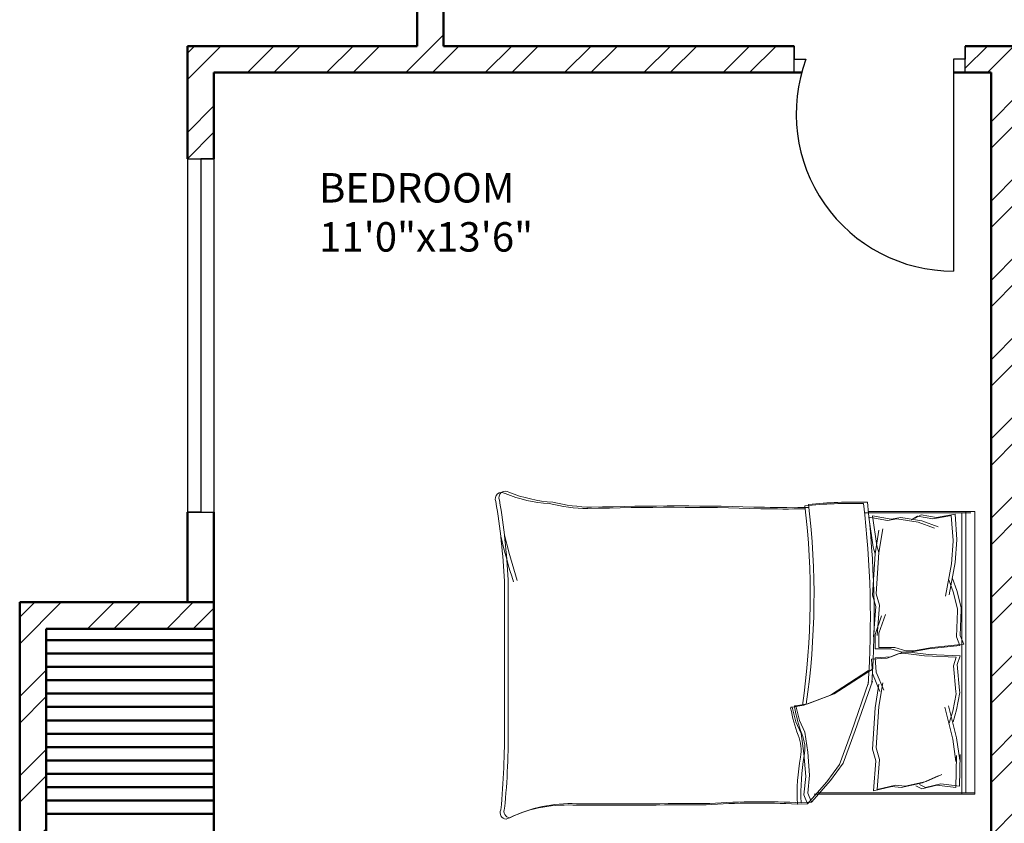
# Model space of a CAD drawing. Units: inches. Extents: x 963 to 2075, y 289 to 2657.
# Tile 2 of 98: x 1091 to 1259, y 1582 to 1718. Entities that reach past the tile are written whole.
import ezdxf

# ---------------------------------------------------------------- set-up
doc = ezdxf.new("R2010")
doc.units = ezdxf.units.IN
for name, color, linetype, lineweight in [('A-AREA-IDEN', 7, 'Continuous', 18), ('A-DOOR', 4, 'Continuous', 25), ('A-FURN', 8, 'Continuous', 18), ('A-GLAZ', 3, 'Continuous', 25), ('A-WALL', 7, 'Continuous', 50), ('A-WALL-PATT', 8, 'Continuous', 13)]:
    doc.layers.add(name, color=color, linetype=linetype, lineweight=lineweight)
doc.styles.get("Standard").update_dxf_attribs({"font": 'arial.ttf'})

# ---------------------------------------------------------------- blocks, each defined once
blk = doc.blocks.new('BED-DOUBLE')
for p, q in [((1236.12, 2450.52), (1254.23, 2450.52)), ((1236.12, 2450.52), (1254.23, 2450.52)), ((1236.76, 2450.75), (1254.87, 2450.75)), ((1236.76, 2450.75), (1254.87, 2450.75)), ((1251.56, 2450.33), (1248.37, 2449.75)), ((1251.56, 2450.33), (1248.37, 2449.75)), ((1251.53, 2450.32), (1251.86, 2446.04)), ((1251.53, 2450.32), (1251.86, 2446.04)), ((1252.7, 2450.52), (1252.7, 2402.73)), ((1252.7, 2450.52), (1252.7, 2402.73)), ((1253.34, 2450.75), (1253.34, 2402.96)), ((1253.34, 2450.75), (1253.34, 2402.96)), ((1254.87, 2450.75), (1254.87, 2402.73)), ((1237.61, 2444.71), (1236.89, 2449.81)), ((1236.89, 2449.81), (1240.07, 2449.23)), ((1237.61, 2444.71), (1236.89, 2449.81)), ((1236.89, 2449.81), (1240.07, 2449.23)), ((1238.25, 2444.94), (1237.53, 2450.04)), ((1237.53, 2450.04), (1240.71, 2449.46)), ((1238.25, 2444.94), (1237.53, 2450.04)), ((1237.53, 2450.04), (1240.71, 2449.46)), ((1240.07, 2449.23), (1241.66, 2449.52)), ((1240.07, 2449.23), (1241.66, 2449.52)), ((1240.71, 2449.46), (1242.3, 2449.75)), ((1240.71, 2449.46), (1242.3, 2449.75)), ((1241.66, 2449.52), (1245.28, 2448.94)), ((1241.66, 2449.52), (1245.28, 2448.94)), ((1242.3, 2449.75), (1245.92, 2449.17)), ((1242.3, 2449.75), (1245.92, 2449.17)), ((1245.13, 2449.96), (1244.12, 2449.38)), ((1245.13, 2449.96), (1244.12, 2449.38)), ((1245.77, 2450.18), (1244.76, 2449.61)), ((1245.77, 2450.18), (1244.76, 2449.61)), ((1247.74, 2449.52), (1245.13, 2449.96)), ((1247.74, 2449.52), (1245.13, 2449.96)), ((1245.28, 2448.94), (1248.02, 2447.93)), ((1245.28, 2448.94), (1248.02, 2447.93)), ((1248.37, 2449.75), (1245.77, 2450.18)), ((1248.37, 2449.75), (1245.77, 2450.18)), ((1245.92, 2449.17), (1248.66, 2448.16)), ((1245.92, 2449.17), (1248.66, 2448.16)), ((1250.92, 2450.1), (1247.74, 2449.52)), ((1250.92, 2450.1), (1247.74, 2449.52)), ((1250.89, 2450.1), (1251.22, 2445.82)), ((1250.89, 2450.1), (1251.22, 2445.82)), ((1238.6, 2447.61), (1237.94, 2443.58)), ((1238.6, 2447.61), (1237.94, 2443.58)), ((1239.24, 2447.84), (1238.58, 2443.81)), ((1239.24, 2447.84), (1238.58, 2443.81)), ((1251.21, 2445.71), (1250.92, 2441.89)), ((1251.21, 2445.71), (1250.92, 2441.89)), ((1251.22, 2445.82), (1251.21, 2445.71)), ((1251.22, 2445.82), (1251.21, 2445.71)), ((1251.84, 2445.94), (1251.56, 2442.11)), ((1251.84, 2445.94), (1251.56, 2442.11)), ((1251.86, 2446.04), (1251.84, 2445.94)), ((1251.86, 2446.04), (1251.84, 2445.94)), ((1237.94, 2443.58), (1237.51, 2436.57)), ((1237.94, 2443.58), (1237.51, 2436.57)), ((1237.94, 2443.58), (1237.61, 2444.71)), ((1237.94, 2443.58), (1237.61, 2444.71)), ((1238.58, 2443.81), (1238.15, 2436.8)), ((1238.58, 2443.81), (1238.15, 2436.8)), ((1238.58, 2443.81), (1238.25, 2444.94)), ((1238.58, 2443.81), (1238.25, 2444.94)), ((1250.92, 2441.89), (1249.9, 2436.39)), ((1250.92, 2441.89), (1249.9, 2436.39)), ((1251.56, 2442.11), (1250.54, 2436.62)), ((1251.56, 2442.11), (1250.54, 2436.62)), ((1174.99, 2438.93), (1174.99, 2414.32)), ((1174.99, 2438.93), (1174.99, 2414.32)), ((1175.63, 2439.16), (1175.63, 2414.55)), ((1175.63, 2439.16), (1175.63, 2414.55)), ((1250.48, 2439.14), (1251.21, 2437.12)), ((1250.48, 2439.14), (1251.21, 2437.12)), ((1251.12, 2439.37), (1251.84, 2437.34)), ((1251.12, 2439.37), (1251.84, 2437.34)), ((1251.21, 2437.12), (1251.93, 2434.22)), ((1251.21, 2437.12), (1251.93, 2434.23)), ((1251.84, 2437.34), (1252.57, 2434.45)), ((1251.84, 2437.34), (1252.57, 2434.45)), ((1237.51, 2436.57), (1238.06, 2434.61)), ((1237.51, 2436.57), (1238.06, 2434.61)), ((1238.15, 2436.8), (1238.7, 2434.84)), ((1238.15, 2436.8), (1238.7, 2434.84)), ((1238.06, 2434.61), (1237.66, 2429.48)), ((1238.06, 2434.61), (1237.66, 2429.48)), ((1238.7, 2434.84), (1238.3, 2429.71)), ((1238.7, 2434.84), (1238.3, 2429.71)), ((1251.93, 2433.9), (1251.78, 2429.46)), ((1251.93, 2433.9), (1251.78, 2429.46)), ((1251.93, 2434.23), (1251.93, 2433.9)), ((1251.93, 2434.22), (1251.93, 2433.9)), ((1252.57, 2434.13), (1252.42, 2429.69)), ((1252.57, 2434.13), (1252.42, 2429.69)), ((1252.57, 2434.45), (1252.57, 2434.13)), ((1252.57, 2434.45), (1252.57, 2434.13)), ((1237.97, 2429.89), (1239.06, 2433.04)), ((1237.97, 2429.89), (1239.06, 2433.04)), ((1238.61, 2430.12), (1239.7, 2433.26)), ((1238.61, 2430.12), (1239.7, 2433.26)), ((1237.97, 2427.43), (1237.97, 2429.89)), ((1237.97, 2427.43), (1237.97, 2429.89)), ((1238.61, 2427.66), (1238.61, 2430.12)), ((1238.61, 2427.66), (1238.61, 2430.12)), ((1251.78, 2429.46), (1252.36, 2428.01)), ((1251.78, 2429.46), (1252.36, 2428.01)), ((1252.42, 2429.69), (1253, 2428.24)), ((1252.42, 2429.69), (1253, 2428.24)), ((1240.65, 2427.43), (1237.97, 2427.43)), ((1240.65, 2427.43), (1237.97, 2427.43)), ((1241.29, 2427.66), (1238.61, 2427.66)), ((1241.29, 2427.66), (1238.61, 2427.66)), ((1242.53, 2426.86), (1240.65, 2427.43)), ((1242.53, 2426.86), (1240.65, 2427.43)), ((1243.17, 2427.08), (1241.29, 2427.66)), ((1243.17, 2427.08), (1241.29, 2427.66)), ((1243.79, 2426.87), (1242.49, 2426.79)), ((1243.79, 2426.87), (1242.49, 2426.79)), ((1243.83, 2426.86), (1242.53, 2426.86)), ((1243.83, 2426.86), (1242.53, 2426.86)), ((1244.47, 2427.08), (1243.17, 2427.08)), ((1244.47, 2427.08), (1243.17, 2427.08)), ((1247, 2426.49), (1243.79, 2426.87)), ((1247, 2426.49), (1243.79, 2426.87)), ((1247.01, 2427.43), (1243.83, 2426.86)), ((1247.01, 2427.43), (1243.83, 2426.86)), ((1247.65, 2427.66), (1244.47, 2427.08)), ((1247.65, 2427.66), (1244.47, 2427.08)), ((1252.36, 2428.01), (1247.01, 2427.43)), ((1252.36, 2428.01), (1247.01, 2427.43)), ((1253, 2428.24), (1247.65, 2427.66)), ((1253, 2428.24), (1247.65, 2427.66)), ((1240.02, 2425.86), (1237.34, 2425.7)), ((1240.02, 2425.86), (1237.34, 2425.7)), ((1237.34, 2425.7), (1237.49, 2423.24)), ((1237.34, 2425.7), (1237.49, 2423.24)), ((1240.66, 2426.09), (1237.98, 2425.93)), ((1240.66, 2426.09), (1237.98, 2425.93)), ((1237.98, 2425.93), (1238.13, 2423.47)), ((1237.98, 2425.93), (1238.13, 2423.47)), ((1241.86, 2426.56), (1240.02, 2425.86)), ((1241.86, 2426.56), (1240.02, 2425.86)), ((1242.49, 2426.79), (1240.66, 2426.09)), ((1242.49, 2426.79), (1240.66, 2426.09)), ((1243.15, 2426.64), (1241.86, 2426.56)), ((1243.15, 2426.64), (1241.86, 2426.56)), ((1246.37, 2426.26), (1243.15, 2426.64)), ((1246.37, 2426.26), (1243.15, 2426.64)), ((1251.74, 2426.02), (1246.37, 2426.26)), ((1251.74, 2426.02), (1246.37, 2426.26)), ((1252.38, 2426.25), (1247, 2426.49)), ((1252.38, 2426.25), (1247, 2426.49)), ((1251.25, 2424.54), (1251.74, 2426.02)), ((1251.25, 2424.54), (1251.74, 2426.02)), ((1251.89, 2424.77), (1252.38, 2426.25)), ((1251.89, 2424.77), (1252.38, 2426.25)), ((1236.85, 2423.74), (1230.36, 2419.55)), ((1236.85, 2423.74), (1230.36, 2419.55)), ((1237.49, 2423.96), (1231, 2419.77)), ((1237.49, 2423.96), (1231, 2419.77)), ((1238.13, 2423.47), (1239.42, 2420.4)), ((1238.13, 2423.47), (1239.42, 2420.4)), ((1251.68, 2420.11), (1251.25, 2424.54)), ((1251.68, 2420.11), (1251.25, 2424.54)), ((1252.31, 2420.34), (1251.89, 2424.77)), ((1252.31, 2420.34), (1251.89, 2424.77)), ((1234.56, 2413.58), (1237.49, 2421.92)), ((1234.56, 2413.58), (1237.49, 2421.92)), ((1237.49, 2423.24), (1238.78, 2420.17)), ((1237.49, 2423.24), (1238.78, 2420.17)), ((1233.92, 2413.35), (1236.85, 2421.69)), ((1233.92, 2413.35), (1236.85, 2421.69)), ((1238.6, 2421.43), (1237.94, 2417.4)), ((1238.6, 2421.43), (1237.94, 2417.4)), ((1239.24, 2421.66), (1238.58, 2417.63)), ((1239.24, 2421.66), (1238.58, 2417.63)), ((1251.7, 2419.79), (1251.68, 2420.11)), ((1251.7, 2419.79), (1251.68, 2420.11)), ((1252.33, 2420.02), (1252.31, 2420.34)), ((1252.33, 2420.02), (1252.31, 2420.34)), ((1230.36, 2419.55), (1225.87, 2417.84)), ((1230.36, 2419.55), (1225.87, 2417.84)), ((1231, 2419.77), (1226.51, 2418.07)), ((1231, 2419.77), (1226.51, 2418.07)), ((1251.15, 2416.86), (1251.7, 2419.79)), ((1251.15, 2416.86), (1251.7, 2419.79)), ((1251.79, 2417.09), (1252.33, 2420.02)), ((1251.79, 2417.09), (1252.33, 2420.02)), ((1225.87, 2417.84), (1223.86, 2417.53)), ((1225.87, 2417.84), (1223.86, 2417.53)), ((1223.86, 2417.53), (1224.47, 2415.05)), ((1223.86, 2417.53), (1224.47, 2415.05)), ((1226.51, 2418.07), (1224.49, 2417.76)), ((1226.51, 2418.07), (1224.49, 2417.76)), ((1224.49, 2417.76), (1225.11, 2415.28)), ((1224.49, 2417.76), (1225.11, 2415.28)), ((1237.94, 2417.4), (1237.51, 2410.39)), ((1237.94, 2417.4), (1237.51, 2410.39)), ((1238.58, 2417.63), (1238.15, 2410.62)), ((1238.58, 2417.63), (1238.15, 2410.62)), ((1251.16, 2412.08), (1249.81, 2417.5)), ((1251.16, 2412.08), (1249.81, 2417.5)), ((1251.8, 2412.31), (1250.45, 2417.73)), ((1251.8, 2412.31), (1250.45, 2417.73)), ((1250.56, 2414.79), (1251.15, 2416.86)), ((1250.56, 2414.79), (1251.15, 2416.86)), ((1251.2, 2415.02), (1251.79, 2417.09)), ((1251.2, 2415.02), (1251.79, 2417.09)), ((1225.11, 2415.28), (1226.04, 2413.27)), ((1225.11, 2415.28), (1226.04, 2413.27)), ((1224.47, 2415.05), (1225.4, 2413.04)), ((1224.47, 2415.05), (1225.4, 2413.04)), ((1232.54, 2408), (1234.56, 2413.58)), ((1232.54, 2408), (1234.56, 2413.58)), ((1225.4, 2413.04), (1225.87, 2409.63)), ((1225.4, 2413.04), (1225.87, 2409.63)), ((1226.04, 2413.27), (1226.51, 2409.86)), ((1226.04, 2413.27), (1226.51, 2409.86)), ((1231.9, 2407.77), (1233.92, 2413.35)), ((1231.9, 2407.78), (1233.92, 2413.35)), ((1251.69, 2408.28), (1251.16, 2412.08)), ((1251.69, 2408.28), (1251.16, 2412.08)), ((1252.33, 2408.51), (1251.8, 2412.31)), ((1252.33, 2408.51), (1251.8, 2412.31)), ((1237.51, 2410.39), (1238.06, 2408.43)), ((1237.51, 2410.39), (1238.06, 2408.43)), ((1238.15, 2410.62), (1238.7, 2408.66)), ((1238.15, 2410.62), (1238.7, 2408.66)), ((1225.87, 2409.63), (1226.18, 2405.76)), ((1225.87, 2409.63), (1226.18, 2405.76)), ((1226.51, 2409.86), (1226.82, 2405.99)), ((1226.51, 2409.86), (1226.82, 2405.99)), ((1238.06, 2408.43), (1237.66, 2403.3)), ((1238.06, 2408.43), (1237.66, 2403.3)), ((1238.7, 2408.66), (1238.3, 2403.52)), ((1238.7, 2408.66), (1238.3, 2403.52)), ((1251.68, 2403.88), (1251.77, 2409.29)), ((1251.68, 2403.88), (1251.77, 2409.28)), ((1251.77, 2409.29), (1251.69, 2408.28)), ((1251.77, 2409.28), (1251.69, 2408.28)), ((1252.31, 2404.11), (1252.41, 2409.51)), ((1252.31, 2404.11), (1252.41, 2409.51)), ((1252.41, 2409.51), (1252.33, 2408.51)), ((1252.41, 2409.51), (1252.33, 2408.51)), ((1229.74, 2404.83), (1231.9, 2407.78)), ((1229.74, 2404.83), (1231.9, 2407.77)), ((1230.38, 2405.06), (1232.54, 2408)), ((1230.38, 2405.06), (1232.54, 2408)), ((1226.18, 2405.76), (1225.87, 2402.66)), ((1226.18, 2405.76), (1225.87, 2402.66)), ((1226.82, 2405.99), (1226.51, 2402.89)), ((1226.82, 2405.99), (1226.51, 2402.89)), ((1227.13, 2401.36), (1230.38, 2405.06)), ((1227.13, 2401.36), (1230.38, 2405.06)), ((1245.98, 2404.69), (1248.65, 2405.87)), ((1245.98, 2404.69), (1248.65, 2405.87)), ((1246.61, 2404.91), (1249.29, 2406.1)), ((1246.61, 2404.91), (1249.29, 2406.09)), ((1226.49, 2401.13), (1229.74, 2404.83)), ((1226.49, 2401.13), (1229.74, 2404.83)), ((1237.66, 2403.3), (1240.8, 2404.07)), ((1237.66, 2403.3), (1240.8, 2404.07)), ((1238.3, 2403.52), (1241.44, 2404.3)), ((1238.3, 2403.52), (1241.44, 2404.3)), ((1240.8, 2404.07), (1242.4, 2403.88)), ((1240.8, 2404.07), (1242.4, 2403.88)), ((1241.44, 2404.3), (1243.04, 2404.11)), ((1241.44, 2404.3), (1243.04, 2404.11)), ((1242.4, 2403.88), (1245.98, 2404.69)), ((1242.4, 2403.88), (1245.98, 2404.69)), ((1243.04, 2404.11), (1246.61, 2404.91)), ((1243.04, 2404.11), (1246.61, 2404.91)), ((1245.89, 2403.67), (1244.85, 2404.18)), ((1245.89, 2403.67), (1244.85, 2404.18)), ((1246.53, 2403.89), (1245.49, 2404.41)), ((1246.53, 2403.89), (1245.49, 2404.41)), ((1248.46, 2404.26), (1245.89, 2403.67)), ((1248.46, 2404.26), (1245.89, 2403.67)), ((1249.1, 2404.49), (1246.53, 2403.89)), ((1249.1, 2404.49), (1246.53, 2403.89)), ((1251.68, 2403.88), (1248.46, 2404.26)), ((1251.68, 2403.88), (1248.46, 2404.26)), ((1252.31, 2404.11), (1249.1, 2404.49)), ((1252.31, 2404.11), (1249.1, 2404.49)), ((1225.87, 2402.66), (1226.49, 2401.13)), ((1225.87, 2402.66), (1226.49, 2401.13)), ((1226.51, 2402.89), (1227.13, 2401.36)), ((1226.51, 2402.89), (1227.13, 2401.36)), ((1254.23, 2402.73), (1227.62, 2402.73)), ((1254.23, 2402.73), (1227.62, 2402.73)), ((1254.87, 2402.96), (1228.26, 2402.96)), ((1254.87, 2402.96), (1228.26, 2402.96)), ((1254.87, 2402.73), (1254.23, 2402.73)), ((1224.74, 2401.05), (1226.49, 2401.13, 3.87)), ((1224.74, 2401.05), (1226.49, 2401.13, 3.87)), ((1225.38, 2401.28), (1227.13, 2401.36, 3.87)), ((1225.38, 2401.28), (1227.13, 2401.36, 3.87))]:
    blk.add_line(p, q)
for centre, radius, start, end in [((1174.51, 2452.91), 1.09, 56.1736, 203.4781), ((1174.51, 2452.91), 1.09, 56.1736, 203.4781), ((1175.15, 2453.14), 1.09, 56.1736, 203.4781), ((1175.15, 2453.14), 1.09, 56.1736, 203.4781), ((1183.96, 2475.65), 23.56, 247.9751, 266.652), ((1183.96, 2475.65), 23.56, 247.9751, 266.652), ((1184.6, 2475.88), 23.56, 247.9751, 266.652), ((1184.6, 2475.88), 23.56, 247.9751, 266.652), ((1053.4, 2432.57), 121.76, 2.9958, 9.4091), ((1053.4, 2432.57), 121.76, 2.9958, 9.4091), ((1054.03, 2432.8), 121.76, 2.9958, 9.4091), ((1054.03, 2432.8), 121.76, 2.9958, 9.4091), ((1189.72, 2480.89), 29.63, 256.0648, 268.9113), ((1189.72, 2480.89), 29.63, 256.0648, 268.9113), ((1190.36, 2481.12), 29.63, 256.0648, 268.9113), ((1190.36, 2481.12), 29.63, 256.0648, 268.9113), ((1234.14, 2368.83), 83.31, 88.7218, 95.604), ((1234.14, 2368.83), 83.31, 88.7218, 95.604), ((1098.56, 2436.47), 129.02, 351.7845, 6.9006), ((1098.56, 2436.47), 129.02, 351.7845, 6.9006), ((1234.78, 2369.06), 83.31, 88.7218, 95.604), ((1234.78, 2369.06), 83.31, 88.7218, 95.604), ((1072.18, 2432.64), 164.97, 356.0865, 6.7821), ((1072.18, 2432.64), 164.97, 356.0865, 6.7821), ((1072.82, 2432.86), 164.97, 356.0865, 6.7821), ((1072.82, 2432.86), 164.97, 356.0865, 6.7821), ((1203.62, 1969.17), 482.31, 88.2277, 91.7185), ((1203.62, 1969.17), 482.31, 88.2277, 91.7185), ((1204.26, 1969.4), 482.31, 88.2277, 91.7185), ((1204.26, 1969.4), 482.31, 88.2277, 91.7185), ((1223.06, 2621.3), 170.11, 268.4762, 271.0082), ((1223.06, 2621.3), 170.11, 268.4762, 271.0082), ((1223.7, 2621.53), 170.11, 268.4762, 271.0082), ((1223.7, 2621.53), 170.11, 268.4762, 271.0082), ((1097.92, 2436.24), 129.02, 351.7845, 6.9006), ((1097.92, 2436.24), 129.02, 351.7845, 6.9006), ((1277.94, 2471.22), 106.46, 193.3832, 197.7053), ((1277.94, 2471.22), 106.46, 193.3832, 197.7053), ((1278.58, 2471.44), 106.46, 193.3832, 197.7053), ((1278.58, 2471.44), 106.46, 193.3832, 197.7053), ((1223.79, 2417.36), 0.185, 70.2464, 181.1377), ((1223.79, 2417.36), 0.185, 70.2464, 181.1377), ((1252.75, 2422.84), 29.65, 190.6617, 199.8806), ((1252.75, 2422.84), 29.65, 190.6617, 199.8806), ((1224.43, 2417.59), 0.185, 70.2464, 181.1377), ((1224.43, 2417.59), 0.185, 70.2464, 181.1377), ((1253.39, 2423.07), 29.65, 190.6617, 199.8806), ((1253.39, 2423.07), 29.65, 190.6617, 199.8806), ((1041.96, 2412.84), 133.04, 354.4998, 0.6351), ((1041.96, 2412.84), 133.04, 354.4998, 0.6351), ((1042.6, 2413.07), 133.04, 354.4998, 0.6351), ((1042.6, 2413.07), 133.04, 354.4998, 0.6351), ((1219.17, 2410.25), 6.22, 348.6608, 23.7384), ((1219.17, 2410.25), 6.22, 348.6608, 23.7384), ((1219.81, 2410.48), 6.22, 348.6608, 23.7384), ((1219.81, 2410.48), 6.22, 348.6608, 23.7384), ((1260.89, 2402.67), 36.18, 169.8763, 182.5657), ((1260.89, 2402.67), 36.18, 169.8763, 182.5657), ((1261.53, 2402.9), 36.18, 169.8763, 182.5657), ((1261.53, 2402.9), 36.18, 169.8763, 182.5657), ((1175.36, 2399.58), 1.1, 152.6588, 266.02), ((1175.36, 2399.58), 1.1, 152.6588, 266.02), ((1176, 2399.81), 1.1, 152.6588, 266.02), ((1176, 2399.81), 1.1, 152.6588, 266.02), ((1185.57, 2377.84), 23.07, 87.4714, 116.4681), ((1185.57, 2377.84), 23.07, 87.4714, 116.4681), ((1186.21, 2378.07), 23.07, 87.4714, 116.4681), ((1186.21, 2378.07), 23.07, 87.4714, 116.4681), ((1186.41, 6962.74), 4561.86, 270.00217, 270.28689), ((1186.41, 6962.74), 4561.86, 270.00217, 270.28689), ((1187.05, 6962.97), 4561.86, 270.00217, 270.28689), ((1187.05, 6962.97), 4561.86, 270.00217, 270.28689), ((1217.92, 2271.73), 129.5, 86.9791, 93.8365), ((1217.92, 2271.73), 129.5, 86.9791, 93.8365), ((1218.56, 2271.96), 129.5, 86.9791, 93.8365), ((1218.56, 2271.96), 129.5, 86.9791, 93.8365)]:
    blk.add_arc(centre, radius, start, end)

msp = doc.modelspace()

# ---------------------------------------------------------------- hatches: boundary and pattern name
at = {"layer": 'A-WALL-PATT'}
h = msp.add_hatch(dxfattribs=at)
h.set_pattern_fill('ANSI32', color=256)
h.paths.add_polyline_path([(1296.92, 2558.32), (1203.92, 2558.32), (1203.92, 2493.82), (1191.53, 2493.82), (1191.53, 2489.32), (1211.06, 2489.32), (1211.06, 2492.02), (1211.06, 2493.82), (1208.42, 2493.82), (1208.42, 2553.82), (1292.42, 2553.82), (1292.42, 2538.86), (1296.92, 2538.86)])
h.paths.add_polyline_path([(1442.42, 2558.32), (1349.42, 2558.32), (1349.42, 2538.94), (1353.92, 2538.94), (1353.92, 2553.82), (1437.92, 2553.82), (1437.92, 2493.82), (1434.54, 2493.82), (1434.54, 2489.32), (1448.31, 2489.32), (1448.31, 2491.57), (1448.31, 2493.82), (1442.42, 2493.82)])
h.paths.add_polyline_path([(1415.55, 2491.57), (1415.55, 2493.82), (1340.94, 2493.82), (1340.94, 2489.32), (1371.92, 2489.32), (1371.92, 2378.32), (1367.6, 2378.32), (1367.6, 2373.82), (1371.92, 2373.82), (1371.92, 2355.19), (1376.42, 2355.19), (1376.42, 2489.32), (1415.55, 2489.32)])
h.paths.add_polyline_path([(1304.94, 2491.57), (1304.94, 2493.82), (1296.92, 2493.82), (1296.92, 2514.86), (1292.42, 2514.86), (1292.42, 2493.82), (1232.81, 2493.82), (1232.81, 2489.32), (1256.42, 2489.32), (1256.42, 2327.32), (1253.71, 2327.32), (1253.71, 2322.82), (1328.42, 2322.82), (1328.42, 2331.15), (1323.92, 2331.15), (1323.92, 2327.32), (1260.92, 2327.32), (1260.92, 2373.82), (1323.92, 2373.82), (1323.92, 2357.81), (1328.42, 2357.81), (1328.42, 2373.82), (1346.01, 2373.82), (1346.01, 2376.07), (1346.01, 2378.32), (1260.92, 2378.32), (1260.92, 2489.32), (1304.94, 2489.32)])
h.paths.add_polyline_path([(1226.65, 2327.32), (1124.42, 2327.32), (1124.42, 2347.45), (1119.92, 2347.45), (1119.92, 2322.82), (1163.42, 2322.82), (1163.42, 2305.43), (1165.67, 2305.43), (1167.92, 2305.43), (1167.92, 2322.82), (1226.65, 2322.82), (1226.65, 2325.07)])
h.paths.add_polyline_path([(1095.92, 2489.32), (1124.42, 2489.32), (1131.53, 2489.32), (1131.53, 2491.57), (1131.53, 2493.82), (1119.92, 2493.82), (1091.42, 2493.82), (1091.42, 2417.32), (1095.92, 2417.32), (1119.92, 2417.32), (1119.92, 2407.45), (1124.42, 2407.45), (1124.42, 2421.82), (1095.92, 2421.82)])
h.paths.add_polyline_path([(1512.92, 2558.32), (1508.42, 2558.32), (1508.42, 2493.82), (1503.4, 2493.82), (1503.4, 2489.32), (1508.42, 2489.32), (1508.42, 2327.32), (1376.42, 2327.32), (1376.42, 2330.27), (1371.92, 2330.27), (1371.92, 2298.74), (1376.42, 2298.74), (1376.42, 2322.82), (1508.42, 2322.82), (1508.42, 2165.32), (1504.26, 2165.32), (1504.26, 2160.82), (1508.42, 2160.82), (1508.42, 2108.32), (1512.92, 2108.32), (1512.92, 2160.82), (1516.18, 2160.82), (1516.18, 2163.07), (1516.18, 2165.32), (1512.92, 2165.32), (1512.92, 2322.82), (1644.92, 2322.82), (1644.92, 2298.74), (1649.42, 2298.74), (1649.42, 2322.82), (1649.42, 2330.94), (1647.17, 2330.94), (1644.92, 2330.94), (1644.92, 2327.32), (1512.92, 2327.32), (1512.92, 2489.32), (1516.76, 2489.32), (1516.76, 2491.57), (1516.76, 2493.82), (1512.92, 2493.82)])
h.paths.add_polyline_path([(1671.92, 2558.32), (1578.92, 2558.32), (1578.92, 2493.82), (1573.53, 2493.82), (1573.53, 2489.32), (1586.54, 2489.32), (1586.54, 2491.57), (1586.54, 2493.82), (1583.42, 2493.82), (1583.42, 2553.82), (1667.42, 2553.82), (1667.42, 2541.11), (1671.92, 2541.11)])
h.paths.add_polyline_path([(1681.26, 2493.82), (1671.92, 2493.82), (1671.92, 2517.11), (1667.42, 2517.11), (1667.42, 2493.82), (1610.22, 2493.82), (1610.22, 2489.32), (1644.92, 2489.32), (1644.92, 2357.87), (1649.42, 2357.87), (1649.42, 2373.82), (1652.2, 2373.82), (1652.2, 2375.83), (1652.2, 2378.32), (1649.42, 2378.32), (1649.42, 2489.32), (1681.26, 2489.32), (1681.26, 2491.57)])
h.paths.add_polyline_path([(1821.92, 2558.32), (1728.92, 2558.32), (1728.92, 2541), (1733.42, 2541), (1733.42, 2553.82), (1817.42, 2553.82), (1817.42, 2493.82), (1813.51, 2493.82), (1813.51, 2489.32), (1830.08, 2489.32), (1830.08, 2491.57), (1830.08, 2493.82), (1821.92, 2493.82)])
h.paths.add_polyline_path([(1794.24, 2493.82), (1717.26, 2493.82), (1717.26, 2489.32), (1760.42, 2489.32), (1760.42, 2378.32), (1674.4, 2378.32), (1674.4, 2373.82), (1692.92, 2373.82), (1692.92, 2356.95), (1697.42, 2356.95), (1697.42, 2373.82), (1760.42, 2373.82), (1760.42, 2327.32), (1697.42, 2327.32), (1697.42, 2333.34), (1692.92, 2333.34), (1692.92, 2322.82), (1768.04, 2322.82), (1768.04, 2325.07), (1768.04, 2327.32), (1764.92, 2327.32), (1764.92, 2489.32), (1794.24, 2489.32)])
h.paths.add_polyline_path([(1733.42, 2517), (1728.92, 2517), (1728.92, 2493.82), (1733.42, 2493.82)], flags=17)
h.paths.add_polyline_path([(1929.92, 2493.82), (1890.08, 2493.82), (1890.08, 2489.32), (1896.92, 2489.32), (1925.42, 2489.32), (1925.42, 2421.82), (1896.92, 2421.82), (1896.92, 2408.32), (1901.42, 2408.32), (1901.42, 2417.32), (1925.42, 2417.32), (1929.92, 2417.32)])
h.paths.add_polyline_path([(1901.42, 2348.32), (1896.92, 2348.32), (1896.92, 2327.32), (1800.42, 2327.32), (1800.42, 2322.82), (1853.42, 2322.82), (1853.42, 2309.45), (1857.92, 2309.45), (1857.92, 2322.82), (1901.42, 2322.82)])
h.paths.add_polyline_path([(1857.92, 2249.45), (1853.42, 2249.45), (1853.42, 2214.82), (1686.31, 2214.82), (1686.31, 2210.32), (1853.42, 2210.32), (1853.42, 2202.13), (1857.92, 2202.13), (1857.92, 2210.32)])
h.paths.add_polyline_path([(1857.92, 2142.13), (1853.42, 2142.13), (1853.42, 2115.42), (1841.42, 2115.42), (1841.42, 2088.53), (1841.42, 2046.95), (1845.92, 2046.95), (1845.92, 2110.92), (1905.92, 2110.92), (1905.92, 2092.52), (1910.42, 2092.52), (1910.42, 2115.42), (1857.92, 2115.42)])
h.paths.add_polyline_path([(1532.44, 1482.34), (1573.46, 1482.34), (1573.46, 1501), (1532.44, 1501)], flags=9)
h.paths.add_polyline_path([(1438.66, 1486.3), (1479.68, 1486.3), (1479.68, 1504.96), (1438.66, 1504.96)], flags=9)
h.paths.add_polyline_path([(1411.22, 1365.31), (1659.14, 1365.31), (1659.14, 1402.4), (1411.22, 1402.4)], flags=9)
h.paths.add_polyline_path([(1185.67, 2296.3), (1248.16, 2296.3), (1248.16, 2314.95), (1185.67, 2314.95)], flags=9)
h.paths.add_polyline_path([(1177.31, 2187.35), (1216.15, 2187.35), (1216.15, 2206.01), (1177.31, 2206.01)], flags=9)
h.paths.add_polyline_path([(1295.1, 1602.08), (1328.26, 1602.08), (1328.26, 1620.74), (1295.1, 1620.74)], flags=9)
h.paths.add_polyline_path([(1525.13, 2005.99), (1558.39, 2005.99), (1558.39, 2024.65), (1525.13, 2024.65)], flags=9)
h.paths.add_polyline_path([(1459.61, 1977.13), (1472.19, 1977.13), (1472.19, 1987.43), (1459.61, 1987.43)], flags=9)
h.paths.add_polyline_path([(1467.81, 2053.68), (1480.02, 2053.68), (1480.02, 2063.98), (1467.81, 2063.98)], flags=9)
h.paths.add_polyline_path([(1555.18, 2119.02), (1584.56, 2119.02), (1584.56, 2137.68), (1555.18, 2137.68)], flags=25)
h.paths.add_polyline_path([(1405.39, 2115.29), (1444.48, 2115.29), (1444.48, 2133.95), (1405.39, 2133.95)], flags=25)
h.paths.add_polyline_path([(1698.48, 2004.26), (1727.69, 2004.26), (1727.69, 2022.92), (1698.48, 2022.92)], flags=9)
h.paths.add_polyline_path([(1612.16, 1972.86), (1629.02, 1972.86), (1629.02, 1983.16), (1612.16, 1983.16)], flags=9)
h.paths.add_polyline_path([(1608.29, 2060.04), (1625.15, 2060.04), (1625.15, 2070.34), (1608.29, 2070.34)], flags=9)
h.paths.add_polyline_path([(1527.95, 1684.4), (1566.79, 1684.4), (1566.79, 1703.06), (1527.95, 1703.06)], flags=9)
h.paths.add_polyline_path([(1422.79, 1683.59), (1461.63, 1683.59), (1461.63, 1702.25), (1422.79, 1702.25)], flags=9)
h.paths.add_polyline_path([(1531.26, 1732.46), (1574.01, 1732.46), (1574.01, 1751.12), (1531.26, 1751.12)], flags=9)
h.paths.add_polyline_path([(1402.87, 1732.85), (1439.8, 1732.85), (1439.8, 1751.5), (1402.87, 1751.5)], flags=9)
h.paths.add_polyline_path([(1243.12, 1923.13), (1281.96, 1923.13), (1281.96, 1941.79), (1243.12, 1941.79)], flags=9)
h.paths.add_polyline_path([(1181.75, 1792.27), (1244.24, 1792.27), (1244.24, 1810.93), (1181.75, 1810.93)], flags=9)
h.paths.add_polyline_path([(1265.82, 1670.3), (1316.07, 1670.3), (1316.07, 1688.96), (1265.82, 1688.96)], flags=9)
h.paths.add_polyline_path([(1140.26, 1676.05), (1179.1, 1676.05), (1179.1, 1694.71), (1140.26, 1694.71)], flags=9)
h.paths.add_polyline_path([(1107.49, 1490.89), (1143.37, 1490.89), (1143.37, 1509.55), (1107.49, 1509.55)], flags=9)
h.paths.add_polyline_path([(1217.58, 1483.9), (1246.74, 1483.9), (1246.74, 1502.56), (1217.58, 1502.56)], flags=9)
h.paths.add_polyline_path([(1389.21, 1486.92), (1418.37, 1486.92), (1418.37, 1505.58), (1389.21, 1505.58)], flags=9)
h.paths.add_polyline_path([(1672.21, 1602.08), (1705.37, 1602.08), (1705.37, 1620.74), (1672.21, 1620.74)], flags=9)
h.paths.add_polyline_path([(1752.08, 1522.64), (1781.24, 1522.64), (1781.24, 1541.3), (1752.08, 1541.3)], flags=9)
h.paths.add_polyline_path([(1848.27, 1491.26), (1884.16, 1491.26), (1884.16, 1509.92), (1848.27, 1509.92)], flags=9)
h.paths.add_polyline_path([(1822.47, 1685.62), (1861.31, 1685.62), (1861.31, 1704.28), (1822.47, 1704.28)], flags=9)
h.paths.add_polyline_path([(1713.19, 1672.23), (1763.44, 1672.23), (1763.44, 1690.89), (1713.19, 1690.89)], flags=9)
h.paths.add_polyline_path([(1736.62, 1790.58), (1799.11, 1790.58), (1799.11, 1809.24), (1736.62, 1809.24)], flags=9)
h.paths.add_polyline_path([(1691.49, 1916.36), (1730.33, 1916.36), (1730.33, 1935.01), (1691.49, 1935.01)], flags=9)
h.paths.add_polyline_path([(1764.87, 1973.92), (1794.31, 1973.92), (1794.31, 1992.58), (1764.87, 1992.58)], flags=9)
h.paths.add_polyline_path([(1767.85, 2034.02), (1797.29, 2034.02), (1797.29, 2052.67), (1767.85, 2052.67)], flags=9)
h.paths.add_polyline_path([(1851.59, 2060.33), (1880.75, 2060.33), (1880.75, 2078.99), (1851.59, 2078.99)], flags=25)
h.paths.add_polyline_path([(1688.49, 2086.87), (1727.33, 2086.87), (1727.33, 2105.53), (1688.49, 2105.53)], flags=9)
h.paths.add_polyline_path([(1537.74, 2293.58), (1580.49, 2293.58), (1580.49, 2312.24), (1537.74, 2312.24)], flags=25)
h.paths.add_polyline_path([(1425.59, 2296.11), (1468.34, 2296.11), (1468.34, 2314.77), (1425.59, 2314.77)], flags=25)
h.paths.add_polyline_path([(1278.52, 2004.18), (1307.72, 2004.18), (1307.72, 2022.84), (1278.52, 2022.84)], flags=9)
h.paths.add_polyline_path([(1193.28, 1973.63), (1222.72, 1973.63), (1222.72, 1992.29), (1193.28, 1992.29)], flags=9)
h.paths.add_polyline_path([(1192.41, 2040.58), (1221.84, 2040.58), (1221.84, 2059.23), (1192.41, 2059.23)], flags=9)
h.paths.add_polyline_path([(1130.6, 1951.39), (1159.76, 1951.39), (1159.76, 1970.05), (1130.6, 1970.05)], flags=9)
h.paths.add_polyline_path([(1132.83, 2052.49), (1161.98, 2052.49), (1161.98, 2071.15), (1132.83, 2071.15)], flags=9)
h.paths.add_polyline_path([(1265.13, 2334.62), (1315.38, 2334.62), (1315.38, 2353.28), (1265.13, 2353.28)], flags=25)
h.paths.add_polyline_path([(1136.74, 2330.79), (1175.58, 2330.79), (1175.58, 2349.44), (1136.74, 2349.44)], flags=9)
h.paths.add_polyline_path([(1287.42, 2417.2), (1320.58, 2417.2), (1320.58, 2435.86), (1287.42, 2435.86)], flags=25)
h.paths.add_polyline_path([(1430.99, 2329.16), (1469.83, 2329.16), (1469.83, 2347.82), (1430.99, 2347.82)], flags=25)
h.paths.add_polyline_path([(1525.42, 2329.21), (1564.26, 2329.21), (1564.26, 2347.87), (1525.42, 2347.87)], flags=25)
h.paths.add_polyline_path([(1684.52, 2382.8), (1717.68, 2382.8), (1717.68, 2401.46), (1684.52, 2401.46)], flags=25)
h.paths.add_polyline_path([(1704.81, 2340.29), (1755.05, 2340.29), (1755.05, 2358.95), (1704.81, 2358.95)], flags=25)
h.paths.add_polyline_path([(1694.11, 2287.76), (1756.6, 2287.76), (1756.6, 2306.41), (1694.11, 2306.41)], flags=9)
h.paths.add_polyline_path([(1815.78, 2329.86), (1854.62, 2329.86), (1854.62, 2348.52), (1815.78, 2348.52)], flags=9)
h.paths.add_polyline_path([(1842.87, 2514.26), (1878.76, 2514.26), (1878.76, 2532.91), (1842.87, 2532.91)], flags=9)
h.paths.add_polyline_path([(1769.51, 2531.45), (1798.67, 2531.45), (1798.67, 2550.1), (1769.51, 2550.1)], flags=25)
h.paths.add_polyline_path([(1594.77, 2518.47), (1623.93, 2518.47), (1623.93, 2537.13), (1594.77, 2537.13)], flags=25)
h.paths.add_polyline_path([(1520.72, 2516.18), (1556.61, 2516.18), (1556.61, 2534.84), (1520.72, 2534.84)], flags=25)
h.paths.add_polyline_path([(1464.46, 2516.69), (1500.34, 2516.69), (1500.34, 2535.35), (1464.46, 2535.35)], flags=25)
h.paths.add_polyline_path([(1365.7, 2528.97), (1394.85, 2528.97), (1394.85, 2547.63), (1365.7, 2547.63)], flags=25)
h.paths.add_polyline_path([(1222.84, 2516.23), (1252, 2516.23), (1252, 2534.89), (1222.84, 2534.89)], flags=25)
h.paths.add_polyline_path([(1104.55, 2509.6), (1140.43, 2509.6), (1140.43, 2528.26), (1104.55, 2528.26)], flags=9)
h = msp.add_hatch(dxfattribs=at)
h.set_pattern_fill('ANSI32', color=256)
h.paths.add_polyline_path([(1335.97, 2212.57), (1335.97, 2214.82), (1167.92, 2214.82), (1167.92, 2245.43), (1163.42, 2245.43), (1163.42, 2210.32), (1163.42, 2194.81), (1167.92, 2194.81), (1167.92, 2210.32), (1335.97, 2210.32)])
h.paths.add_polyline_path([(1532.44, 1482.34), (1573.46, 1482.34), (1573.46, 1501), (1532.44, 1501)], flags=9)
h.paths.add_polyline_path([(1438.66, 1486.3), (1479.68, 1486.3), (1479.68, 1504.96), (1438.66, 1504.96)], flags=9)
h.paths.add_polyline_path([(1411.22, 1365.31), (1659.14, 1365.31), (1659.14, 1402.4), (1411.22, 1402.4)], flags=9)
h.paths.add_polyline_path([(1185.67, 2296.3), (1248.16, 2296.3), (1248.16, 2314.95), (1185.67, 2314.95)], flags=9)
h.paths.add_polyline_path([(1177.31, 2187.35), (1216.15, 2187.35), (1216.15, 2206.01), (1177.31, 2206.01)], flags=9)
h.paths.add_polyline_path([(1295.1, 1602.08), (1328.26, 1602.08), (1328.26, 1620.74), (1295.1, 1620.74)], flags=9)
h.paths.add_polyline_path([(1525.13, 2005.99), (1558.39, 2005.99), (1558.39, 2024.65), (1525.13, 2024.65)], flags=9)
h.paths.add_polyline_path([(1459.61, 1977.13), (1472.19, 1977.13), (1472.19, 1987.43), (1459.61, 1987.43)], flags=9)
h.paths.add_polyline_path([(1467.81, 2053.68), (1480.02, 2053.68), (1480.02, 2063.98), (1467.81, 2063.98)], flags=9)
h.paths.add_polyline_path([(1555.18, 2119.02), (1584.56, 2119.02), (1584.56, 2137.68), (1555.18, 2137.68)], flags=9)
h.paths.add_polyline_path([(1405.39, 2115.29), (1444.48, 2115.29), (1444.48, 2133.95), (1405.39, 2133.95)], flags=9)
h.paths.add_polyline_path([(1698.48, 2004.26), (1727.69, 2004.26), (1727.69, 2022.92), (1698.48, 2022.92)], flags=9)
h.paths.add_polyline_path([(1612.16, 1972.86), (1629.02, 1972.86), (1629.02, 1983.16), (1612.16, 1983.16)], flags=9)
h.paths.add_polyline_path([(1608.29, 2060.04), (1625.15, 2060.04), (1625.15, 2070.34), (1608.29, 2070.34)], flags=9)
h.paths.add_polyline_path([(1527.95, 1684.4), (1566.79, 1684.4), (1566.79, 1703.06), (1527.95, 1703.06)], flags=9)
h.paths.add_polyline_path([(1422.79, 1683.59), (1461.63, 1683.59), (1461.63, 1702.25), (1422.79, 1702.25)], flags=9)
h.paths.add_polyline_path([(1531.26, 1732.46), (1574.01, 1732.46), (1574.01, 1751.12), (1531.26, 1751.12)], flags=9)
h.paths.add_polyline_path([(1402.87, 1732.85), (1439.8, 1732.85), (1439.8, 1751.5), (1402.87, 1751.5)], flags=9)
h.paths.add_polyline_path([(1243.12, 1923.13), (1281.96, 1923.13), (1281.96, 1941.79), (1243.12, 1941.79)], flags=9)
h.paths.add_polyline_path([(1181.75, 1792.27), (1244.24, 1792.27), (1244.24, 1810.93), (1181.75, 1810.93)], flags=9)
h.paths.add_polyline_path([(1265.82, 1670.3), (1316.07, 1670.3), (1316.07, 1688.96), (1265.82, 1688.96)], flags=9)
h.paths.add_polyline_path([(1140.26, 1676.05), (1179.1, 1676.05), (1179.1, 1694.71), (1140.26, 1694.71)], flags=9)
h.paths.add_polyline_path([(1107.49, 1490.89), (1143.37, 1490.89), (1143.37, 1509.55), (1107.49, 1509.55)], flags=9)
h.paths.add_polyline_path([(1217.58, 1483.9), (1246.74, 1483.9), (1246.74, 1502.56), (1217.58, 1502.56)], flags=9)
h.paths.add_polyline_path([(1389.21, 1486.92), (1418.37, 1486.92), (1418.37, 1505.58), (1389.21, 1505.58)], flags=9)
h.paths.add_polyline_path([(1672.21, 1602.08), (1705.37, 1602.08), (1705.37, 1620.74), (1672.21, 1620.74)], flags=9)
h.paths.add_polyline_path([(1752.08, 1522.64), (1781.24, 1522.64), (1781.24, 1541.3), (1752.08, 1541.3)], flags=9)
h.paths.add_polyline_path([(1848.27, 1491.26), (1884.16, 1491.26), (1884.16, 1509.92), (1848.27, 1509.92)], flags=9)
h.paths.add_polyline_path([(1822.47, 1685.62), (1861.31, 1685.62), (1861.31, 1704.28), (1822.47, 1704.28)], flags=9)
h.paths.add_polyline_path([(1713.19, 1672.23), (1763.44, 1672.23), (1763.44, 1690.89), (1713.19, 1690.89)], flags=9)
h.paths.add_polyline_path([(1736.62, 1790.58), (1799.11, 1790.58), (1799.11, 1809.24), (1736.62, 1809.24)], flags=9)
h.paths.add_polyline_path([(1691.49, 1916.36), (1730.33, 1916.36), (1730.33, 1935.01), (1691.49, 1935.01)], flags=9)
h.paths.add_polyline_path([(1764.87, 1973.92), (1794.31, 1973.92), (1794.31, 1992.58), (1764.87, 1992.58)], flags=9)
h.paths.add_polyline_path([(1767.85, 2034.02), (1797.29, 2034.02), (1797.29, 2052.67), (1767.85, 2052.67)], flags=9)
h.paths.add_polyline_path([(1851.59, 2060.33), (1880.75, 2060.33), (1880.75, 2078.99), (1851.59, 2078.99)], flags=9)
h.paths.add_polyline_path([(1688.49, 2086.87), (1727.33, 2086.87), (1727.33, 2105.53), (1688.49, 2105.53)], flags=9)
h.paths.add_polyline_path([(1537.74, 2293.58), (1580.49, 2293.58), (1580.49, 2312.24), (1537.74, 2312.24)], flags=9)
h.paths.add_polyline_path([(1425.59, 2296.11), (1468.34, 2296.11), (1468.34, 2314.77), (1425.59, 2314.77)], flags=9)
h.paths.add_polyline_path([(1278.52, 2004.18), (1307.72, 2004.18), (1307.72, 2022.84), (1278.52, 2022.84)], flags=9)
h.paths.add_polyline_path([(1193.28, 1973.63), (1222.72, 1973.63), (1222.72, 1992.29), (1193.28, 1992.29)], flags=9)
h.paths.add_polyline_path([(1192.41, 2040.58), (1221.84, 2040.58), (1221.84, 2059.23), (1192.41, 2059.23)], flags=9)
h.paths.add_polyline_path([(1130.6, 1951.39), (1159.76, 1951.39), (1159.76, 1970.05), (1130.6, 1970.05)], flags=9)
h.paths.add_polyline_path([(1132.83, 2052.49), (1161.98, 2052.49), (1161.98, 2071.15), (1132.83, 2071.15)], flags=9)
h.paths.add_polyline_path([(1265.13, 2334.62), (1315.38, 2334.62), (1315.38, 2353.28), (1265.13, 2353.28)], flags=9)
h.paths.add_polyline_path([(1136.74, 2330.79), (1175.58, 2330.79), (1175.58, 2349.44), (1136.74, 2349.44)], flags=9)
h.paths.add_polyline_path([(1287.42, 2417.2), (1320.58, 2417.2), (1320.58, 2435.86), (1287.42, 2435.86)], flags=9)
h.paths.add_polyline_path([(1430.99, 2329.16), (1469.83, 2329.16), (1469.83, 2347.82), (1430.99, 2347.82)], flags=9)
h.paths.add_polyline_path([(1525.42, 2329.21), (1564.26, 2329.21), (1564.26, 2347.87), (1525.42, 2347.87)], flags=9)
h.paths.add_polyline_path([(1684.52, 2382.8), (1717.68, 2382.8), (1717.68, 2401.46), (1684.52, 2401.46)], flags=9)
h.paths.add_polyline_path([(1704.81, 2340.29), (1755.05, 2340.29), (1755.05, 2358.95), (1704.81, 2358.95)], flags=9)
h.paths.add_polyline_path([(1694.11, 2287.76), (1756.6, 2287.76), (1756.6, 2306.41), (1694.11, 2306.41)], flags=9)
h.paths.add_polyline_path([(1815.78, 2329.86), (1854.62, 2329.86), (1854.62, 2348.52), (1815.78, 2348.52)], flags=9)
h.paths.add_polyline_path([(1842.87, 2514.26), (1878.76, 2514.26), (1878.76, 2532.91), (1842.87, 2532.91)], flags=9)
h.paths.add_polyline_path([(1769.51, 2531.45), (1798.67, 2531.45), (1798.67, 2550.1), (1769.51, 2550.1)], flags=9)
h.paths.add_polyline_path([(1594.77, 2518.47), (1623.93, 2518.47), (1623.93, 2537.13), (1594.77, 2537.13)], flags=9)
h.paths.add_polyline_path([(1520.72, 2516.18), (1556.61, 2516.18), (1556.61, 2534.84), (1520.72, 2534.84)], flags=9)
h.paths.add_polyline_path([(1464.46, 2516.69), (1500.34, 2516.69), (1500.34, 2535.35), (1464.46, 2535.35)], flags=9)
h.paths.add_polyline_path([(1365.7, 2528.97), (1394.85, 2528.97), (1394.85, 2547.63), (1365.7, 2547.63)], flags=9)
h.paths.add_polyline_path([(1222.84, 2516.23), (1252, 2516.23), (1252, 2534.89), (1222.84, 2534.89)], flags=9)
h.paths.add_polyline_path([(1104.55, 2509.6), (1140.43, 2509.6), (1140.43, 2528.26), (1104.55, 2528.26)], flags=9)
h = msp.add_hatch(dxfattribs=at)
h.set_pattern_fill('ANSI32', color=256)
h.paths.add_polyline_path([(1473.61, 2163.07), (1473.61, 2165.32), (1376.42, 2165.32), (1376.42, 2227.98), (1371.92, 2227.98), (1371.92, 2214.82), (1368.41, 2214.82), (1368.41, 2210.32), (1371.92, 2210.32), (1371.92, 2160.82), (1395.92, 2160.82), (1395.92, 2090.32), (1217.34, 2090.32), (1217.34, 2085.82), (1395.92, 2085.82), (1458.92, 2085.82), (1458.92, 2108.32), (1454.42, 2108.32), (1454.42, 2090.32), (1400.42, 2090.32), (1400.42, 2160.82), (1473.61, 2160.82)])
h.paths.add_polyline_path([(1649.42, 2210.32), (1653.23, 2210.32), (1653.23, 2214.82), (1649.42, 2214.82), (1649.42, 2227.98), (1644.92, 2227.98), (1644.92, 2165.32), (1550.1, 2165.32), (1550.1, 2160.82), (1620.92, 2160.82), (1620.92, 2112.82), (1555.45, 2112.82), (1555.45, 2108.32), (1584.33, 2108.32), (1584.33, 2084.92), (1588.83, 2084.92), (1588.83, 2108.32), (1625.42, 2108.32), (1667.95, 2108.32), (1667.95, 2022.67), (1588.83, 2022.67), (1588.83, 2047.41), (1584.33, 2047.41), (1584.33, 1996), (1588.83, 1996), (1588.83, 2018.32), (1667.95, 2018.17), (1667.95, 1928.32), (1625.42, 1928.32), (1625.42, 1923.82), (1672.45, 1923.82), (1672.45, 1928.32), (1672.45, 1946.66), (1785.45, 1946.66), (1785.45, 1951.16), (1743.03, 1951.16), (1743.03, 2017.92), (1841.42, 2017.92), (1841.42, 2014.77), (1845.92, 2014.77), (1845.92, 2017.92), (1905.92, 2017.92), (1905.92, 1987.51), (1910.42, 1987.51), (1910.42, 2022.42), (1910.42, 2068.52), (1905.92, 2068.52), (1905.92, 2022.42), (1845.92, 2022.42), (1845.92, 2025.85), (1843.67, 2025.85), (1841.42, 2025.85), (1841.42, 2022.42), (1743.03, 2022.42), (1743.03, 2084.03), (1768.45, 2084.03), (1785.45, 2084.03), (1785.45, 2088.53), (1672.45, 2088.53), (1672.45, 2112.82), (1667.95, 2112.82), (1625.42, 2112.82), (1625.42, 2160.82), (1649.42, 2160.82)])
h.paths.add_polyline_path([(1672.45, 2084.03), (1738.53, 2084.03), (1738.53, 1951.16), (1672.45, 1951.16)], flags=16)
h.paths.add_polyline_path([(1672.45, 2084.03), (1738.53, 2084.03), (1705.49, 2017.6)], flags=0)
h.paths.add_polyline_path([(1262.77, 2085.82), (1258.27, 2085.82), (1258.27, 2023.28), (1184.42, 2023.28), (1184.42, 2018.78), (1258.27, 2018.78), (1258.27, 1950.82), (1262.77, 1950.82)])
h.paths.add_polyline_path([(1312.27, 2085.82), (1307.77, 2085.82), (1307.77, 1950.82), (1312.27, 1950.82)])
h.paths.add_polyline_path([(1458.92, 1950.82), (1395.92, 1950.82), (1216.57, 1950.82), (1216.57, 1946.32), (1346.42, 1946.32), (1395.92, 1946.32), (1395.92, 1875.82), (1371.92, 1875.82), (1371.92, 1826.32), (1368.93, 1826.32), (1368.93, 1821.82), (1371.92, 1821.82), (1371.92, 1813.62), (1376.42, 1813.62), (1376.42, 1871.32), (1474.5, 1871.32), (1474.5, 1873.57), (1474.5, 1875.82), (1400.42, 1875.82), (1400.42, 1946.32), (1454.42, 1946.32), (1454.42, 1928.32), (1458.92, 1928.32)])
h.paths.add_polyline_path([(1184.42, 2120.78), (1167.92, 2120.78), (1167.92, 2134.81), (1165.67, 2134.81), (1163.42, 2134.81), (1163.42, 2120.78), (1119.92, 2120.78), (1119.92, 2098.1), (1124.42, 2098.1), (1124.42, 2116.28), (1167.92, 2116.28), (1179.92, 2116.28), (1179.92, 2045.92), (1184.42, 2045.92), (1184.42, 2090.32), (1184.42, 2116.28)])
h.paths.add_polyline_path([(1124.42, 2018.78), (1179.92, 2018.78), (1179.92, 2016.29), (1184.42, 2016.29), (1184.42, 2023.28), (1184.42, 2026.59), (1182.17, 2026.59), (1179.92, 2026.59), (1179.92, 2023.28), (1124.42, 2023.28), (1124.42, 2074.1), (1119.92, 2074.1), (1119.92, 2018.78), (1119.92, 1979.63), (1124.42, 1979.63)])
h.paths.add_polyline_path([(1184.42, 1925.78), (1184.42, 1946.32), (1184.42, 1996.07), (1182.17, 1996.07), (1179.92, 1996.07), (1179.92, 1925.78), (1124.42, 1925.78), (1124.42, 1955.63), (1119.92, 1955.5), (1119.92, 1921.28), (1158.92, 1921.28), (1158.92, 1909.98), (1163.42, 1909.98), (1163.42, 1921.28), (1184.42, 1921.28)])
h.paths.add_polyline_path([(1341.45, 1826.32), (1163.42, 1826.32), (1163.42, 1849.98), (1158.92, 1849.98), (1158.92, 1821.82), (1158.92, 1804.03), (1163.42, 1804.03), (1163.42, 1821.82), (1341.45, 1821.82)])
h.paths.add_polyline_path([(1222.98, 1713.82), (1163.42, 1713.82), (1163.42, 1744.03), (1161.17, 1744.03), (1158.92, 1744.03), (1158.92, 1713.82), (1119.92, 1713.82), (1119.92, 1694.65), (1124.42, 1694.65), (1124.42, 1709.32), (1158.92, 1709.32), (1222.98, 1709.32)])
h.paths.add_polyline_path([(1328.42, 1713.82), (1252.04, 1713.82), (1252.04, 1711.57), (1252.04, 1709.32), (1256.42, 1709.32), (1256.42, 1547.32), (1232.94, 1547.32), (1232.94, 1545.07), (1232.94, 1542.82), (1292.42, 1542.82), (1292.42, 1527.63), (1296.92, 1527.63), (1296.92, 1542.82), (1299.46, 1542.82), (1299.46, 1547.32), (1260.92, 1547.32), (1260.92, 1658.32), (1343.66, 1658.32), (1343.66, 1660.57), (1343.66, 1662.82), (1328.42, 1662.82), (1328.42, 1676.59), (1327.4, 1676.59), (1323.92, 1676.59), (1323.92, 1662.82), (1260.92, 1662.82), (1260.92, 1709.32), (1323.92, 1709.32), (1323.92, 1699.85), (1328.42, 1699.85)])
h.paths.add_polyline_path([(1649.42, 1875.82), (1625.42, 1875.82), (1625.42, 1928.32), (1620.92, 1928.32), (1588.83, 1928.32), (1588.83, 1950.59), (1584.33, 1950.59), (1584.33, 1928.32), (1555.45, 1928.32), (1555.45, 1923.82), (1620.92, 1923.82), (1620.92, 1875.82), (1548.95, 1875.82), (1548.95, 1873.57), (1548.95, 1871.32), (1644.92, 1871.32), (1644.92, 1813.62), (1649.42, 1813.62), (1649.42, 1821.82), (1652.04, 1821.82), (1652.04, 1824.07), (1652.04, 1826.32), (1649.42, 1826.32)])
h.paths.add_polyline_path([(1512.92, 1871.32), (1516.48, 1871.32), (1516.48, 1875.82), (1512.92, 1875.82), (1512.92, 1923.82), (1512.92, 1928.32), (1512.92, 1930.83), (1508.42, 1930.83), (1508.42, 1875.82), (1504.41, 1875.82), (1504.41, 1871.32), (1508.42, 1871.32), (1508.42, 1713.82), (1376.42, 1713.82), (1376.42, 1743.32), (1371.92, 1743.32), (1371.92, 1709.32), (1371.92, 1706.01), (1376.42, 1706.01), (1376.42, 1709.32), (1508.42, 1709.32), (1508.42, 1547.32), (1501.87, 1547.32), (1501.87, 1542.82), (1508.42, 1542.82), (1508.42, 1482.82), (1508.42, 1436.32), (1512.92, 1436.32), (1512.92, 1542.82), (1519.32, 1542.82), (1519.32, 1545.07), (1519.32, 1547.32), (1512.92, 1547.32), (1512.92, 1709.32), (1644.92, 1709.32), (1644.92, 1707.55), (1649.42, 1707.55), (1649.42, 1709.32), (1649.42, 1743.32), (1644.92, 1743.32), (1644.92, 1713.82), (1512.92, 1713.82)])
h.paths.add_polyline_path([(1129.88, 1545.07), (1129.88, 1547.32), (1124.42, 1547.32), (1095.92, 1547.32), (1095.92, 1614.82), (1124.42, 1614.82), (1124.42, 1619.32), (1095.92, 1619.32), (1091.42, 1619.32), (1091.42, 1542.82), (1095.92, 1542.82), (1119.92, 1542.82), (1129.88, 1542.82)])
h.paths.add_polyline_path([(1208.42, 1542.82), (1211.74, 1542.82), (1211.74, 1547.32), (1198.85, 1547.32), (1198.85, 1542.82), (1203.92, 1542.82), (1203.92, 1478.32), (1208.42, 1478.32), (1296.92, 1478.32), (1296.92, 1503.63), (1292.42, 1503.63), (1292.42, 1482.82), (1208.42, 1482.82)])
h.paths.add_polyline_path([(1430.42, 1542.82), (1435.7, 1542.82), (1435.7, 1545.07), (1435.7, 1547.32), (1422.66, 1547.32), (1422.66, 1545.07), (1422.66, 1542.82), (1425.92, 1542.82), (1425.92, 1482.86), (1341.92, 1482.86), (1341.92, 1502.73), (1337.42, 1502.73), (1337.42, 1478.36), (1425.92, 1478.36), (1425.92, 1440.82), (1425.92, 1436.32), (1430.42, 1436.32)])
h.paths.add_polyline_path([(1698.48, 2004.26), (1727.69, 2004.26), (1727.69, 2022.92), (1698.48, 2022.92)], flags=8)

# ---------------------------------------------------------------- linework, layer by layer
at = {"layer": 'A-DOOR'}
for p, q in [((1222.98, 1709.32), (1222.98, 1713.82)), ((1222.98, 1713.82), (1222.98, 1711.57)), ((1252.04, 1709.32), (1252.04, 1713.82)), ((1252.04, 1713.82), (1252.04, 1711.57)), ((1222.98, 1711.57), (1224.98, 1711.57)), ((1252.04, 1711.57), (1250.04, 1711.57)), ((1250.04, 1711.57), (1250.04, 1675.57))]:
    msp.add_line(p, q, dxfattribs=at)
msp.add_arc((1250.04, 1702.29), 26.72, 159.6854, 270, dxfattribs=at)
at = {"layer": 'A-GLAZ'}
for p, q in [((1119.92, 1694.65), (1124.42, 1694.65)), ((1119.92, 1694.65), (1119.92, 1634.65)), ((1124.42, 1694.65), (1122.17, 1694.65)), ((1122.17, 1694.65), (1122.17, 1634.65)), ((1124.42, 1694.65), (1124.42, 1634.65)), ((1122.17, 1634.65), (1119.92, 1634.65)), ((1119.92, 1634.65), (1124.42, 1634.65))]:
    msp.add_line(p, q, dxfattribs=at)
at = {"layer": 'A-WALL'}
for p, q in [((1158.92, 1713.82), (1158.92, 1744.03)), ((1163.42, 1744.03), (1163.42, 1713.82)), ((1158.92, 1713.82), (1119.92, 1713.82)), ((1119.92, 1713.82), (1119.92, 1694.65)), ((1163.42, 1713.82), (1222.98, 1713.82)), ((1252.04, 1713.82), (1328.42, 1713.82)), ((1158.92, 1709.32), (1124.42, 1709.32)), ((1124.42, 1709.32), (1124.42, 1694.65)), ((1124.42, 1709.32), (1124.42, 1694.65)), ((1224.26, 1709.32), (1158.92, 1709.32)), ((1256.42, 1709.32), (1250.04, 1709.32)), ((1256.42, 1709.32), (1256.42, 1547.32)), ((1119.92, 1634.65), (1119.92, 1619.32)), ((1124.42, 1634.65), (1124.42, 1547.32)), ((1124.42, 1634.65), (1124.42, 1547.32)), ((1095.92, 1619.32), (1091.42, 1619.32)), ((1091.42, 1619.32), (1091.42, 1542.82)), ((1124.42, 1619.32), (1095.92, 1619.32)), ((1124.42, 1614.82), (1124.42, 1619.32)), ((1095.92, 1547.32), (1095.92, 1614.82)), ((1095.92, 1614.82), (1124.42, 1614.82)), ((1124.42, 1612.9), (1095.92, 1612.9)), ((1124.42, 1610.63), (1095.92, 1610.63)), ((1124.42, 1608.36), (1095.92, 1608.36)), ((1124.42, 1606.08), (1095.92, 1606.08)), ((1124.42, 1603.81), (1095.92, 1603.81)), ((1124.42, 1601.53), (1095.92, 1601.53)), ((1124.42, 1599.26), (1095.92, 1599.26)), ((1124.42, 1596.99), (1095.92, 1596.99)), ((1124.42, 1594.71), (1095.92, 1594.71)), ((1124.42, 1592.44), (1095.92, 1592.44)), ((1124.42, 1590.17), (1095.92, 1590.17)), ((1124.42, 1587.89), (1095.92, 1587.89)), ((1124.42, 1585.62), (1095.92, 1585.62)), ((1124.42, 1583.35), (1095.92, 1583.35))]:
    msp.add_line(p, q, dxfattribs=at)

# ---------------------------------------------------------------- block references
at = {"layer": 'A-FURN'}
msp.add_blockref('BED-DOUBLE', (-1.23, -816.03), dxfattribs=at)

# ---------------------------------------------------------------- texts
at = {"layer": 'A-AREA-IDEN', "insert": (1142.27, 1692.23), "char_height": 5, "attachment_point": 1}
msp.add_mtext_dynamic_manual_height_columns('BEDROOM\\P11\'0"x13\'6"', width=174.7799, gutter_width=12.5, heights=[0], dxfattribs=at)

doc.saveas('drawing.dxf')
